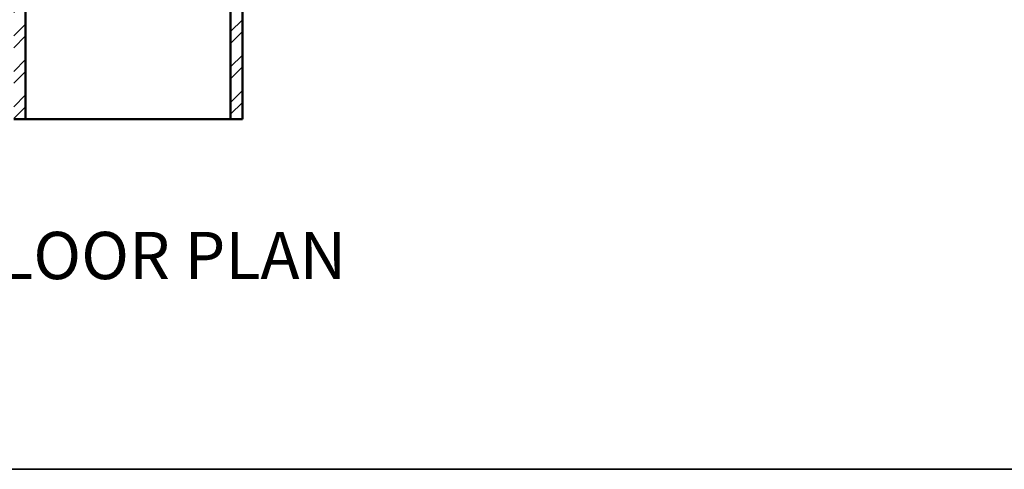
# Model space of a CAD drawing. Units: inches. Extents: x 963 to 2075, y 289 to 2657.
# Tile 30 of 98: x 1511 to 1885, y 1303 to 1474. Entities that reach past the tile are written whole.
import ezdxf

# ---------------------------------------------------------------- set-up
doc = ezdxf.new("R2010")
doc.units = ezdxf.units.IN
for name, color, linetype, lineweight in [('A-ANNO-TEXT', 7, 'Continuous', 25), ('A-ANNO-TTLB', 7, 'Continuous', 35), ('A-WALL', 7, 'Continuous', 50), ('A-WALL-PATT', 8, 'Continuous', 13)]:
    doc.layers.add(name, color=color, linetype=linetype, lineweight=lineweight)
doc.styles.get("Standard").update_dxf_attribs({"font": 'arial.ttf'})

msp = doc.modelspace()

# ---------------------------------------------------------------- hatches: boundary and pattern name
at = {"layer": 'A-WALL-PATT'}
h = msp.add_hatch(dxfattribs=at)
h.set_pattern_fill('ANSI32', color=256)
h.paths.add_polyline_path([(1296.92, 2558.32), (1203.92, 2558.32), (1203.92, 2493.82), (1191.53, 2493.82), (1191.53, 2489.32), (1211.06, 2489.32), (1211.06, 2492.02), (1211.06, 2493.82), (1208.42, 2493.82), (1208.42, 2553.82), (1292.42, 2553.82), (1292.42, 2538.86), (1296.92, 2538.86)])
h.paths.add_polyline_path([(1442.42, 2558.32), (1349.42, 2558.32), (1349.42, 2538.94), (1353.92, 2538.94), (1353.92, 2553.82), (1437.92, 2553.82), (1437.92, 2493.82), (1434.54, 2493.82), (1434.54, 2489.32), (1448.31, 2489.32), (1448.31, 2491.57), (1448.31, 2493.82), (1442.42, 2493.82)])
h.paths.add_polyline_path([(1415.55, 2491.57), (1415.55, 2493.82), (1340.94, 2493.82), (1340.94, 2489.32), (1371.92, 2489.32), (1371.92, 2378.32), (1367.6, 2378.32), (1367.6, 2373.82), (1371.92, 2373.82), (1371.92, 2355.19), (1376.42, 2355.19), (1376.42, 2489.32), (1415.55, 2489.32)])
h.paths.add_polyline_path([(1304.94, 2491.57), (1304.94, 2493.82), (1296.92, 2493.82), (1296.92, 2514.86), (1292.42, 2514.86), (1292.42, 2493.82), (1232.81, 2493.82), (1232.81, 2489.32), (1256.42, 2489.32), (1256.42, 2327.32), (1253.71, 2327.32), (1253.71, 2322.82), (1328.42, 2322.82), (1328.42, 2331.15), (1323.92, 2331.15), (1323.92, 2327.32), (1260.92, 2327.32), (1260.92, 2373.82), (1323.92, 2373.82), (1323.92, 2357.81), (1328.42, 2357.81), (1328.42, 2373.82), (1346.01, 2373.82), (1346.01, 2376.07), (1346.01, 2378.32), (1260.92, 2378.32), (1260.92, 2489.32), (1304.94, 2489.32)])
h.paths.add_polyline_path([(1226.65, 2327.32), (1124.42, 2327.32), (1124.42, 2347.45), (1119.92, 2347.45), (1119.92, 2322.82), (1163.42, 2322.82), (1163.42, 2305.43), (1165.67, 2305.43), (1167.92, 2305.43), (1167.92, 2322.82), (1226.65, 2322.82), (1226.65, 2325.07)])
h.paths.add_polyline_path([(1095.92, 2489.32), (1124.42, 2489.32), (1131.53, 2489.32), (1131.53, 2491.57), (1131.53, 2493.82), (1119.92, 2493.82), (1091.42, 2493.82), (1091.42, 2417.32), (1095.92, 2417.32), (1119.92, 2417.32), (1119.92, 2407.45), (1124.42, 2407.45), (1124.42, 2421.82), (1095.92, 2421.82)])
h.paths.add_polyline_path([(1512.92, 2558.32), (1508.42, 2558.32), (1508.42, 2493.82), (1503.4, 2493.82), (1503.4, 2489.32), (1508.42, 2489.32), (1508.42, 2327.32), (1376.42, 2327.32), (1376.42, 2330.27), (1371.92, 2330.27), (1371.92, 2298.74), (1376.42, 2298.74), (1376.42, 2322.82), (1508.42, 2322.82), (1508.42, 2165.32), (1504.26, 2165.32), (1504.26, 2160.82), (1508.42, 2160.82), (1508.42, 2108.32), (1512.92, 2108.32), (1512.92, 2160.82), (1516.18, 2160.82), (1516.18, 2163.07), (1516.18, 2165.32), (1512.92, 2165.32), (1512.92, 2322.82), (1644.92, 2322.82), (1644.92, 2298.74), (1649.42, 2298.74), (1649.42, 2322.82), (1649.42, 2330.94), (1647.17, 2330.94), (1644.92, 2330.94), (1644.92, 2327.32), (1512.92, 2327.32), (1512.92, 2489.32), (1516.76, 2489.32), (1516.76, 2491.57), (1516.76, 2493.82), (1512.92, 2493.82)])
h.paths.add_polyline_path([(1671.92, 2558.32), (1578.92, 2558.32), (1578.92, 2493.82), (1573.53, 2493.82), (1573.53, 2489.32), (1586.54, 2489.32), (1586.54, 2491.57), (1586.54, 2493.82), (1583.42, 2493.82), (1583.42, 2553.82), (1667.42, 2553.82), (1667.42, 2541.11), (1671.92, 2541.11)])
h.paths.add_polyline_path([(1681.26, 2493.82), (1671.92, 2493.82), (1671.92, 2517.11), (1667.42, 2517.11), (1667.42, 2493.82), (1610.22, 2493.82), (1610.22, 2489.32), (1644.92, 2489.32), (1644.92, 2357.87), (1649.42, 2357.87), (1649.42, 2373.82), (1652.2, 2373.82), (1652.2, 2375.83), (1652.2, 2378.32), (1649.42, 2378.32), (1649.42, 2489.32), (1681.26, 2489.32), (1681.26, 2491.57)])
h.paths.add_polyline_path([(1821.92, 2558.32), (1728.92, 2558.32), (1728.92, 2541), (1733.42, 2541), (1733.42, 2553.82), (1817.42, 2553.82), (1817.42, 2493.82), (1813.51, 2493.82), (1813.51, 2489.32), (1830.08, 2489.32), (1830.08, 2491.57), (1830.08, 2493.82), (1821.92, 2493.82)])
h.paths.add_polyline_path([(1794.24, 2493.82), (1717.26, 2493.82), (1717.26, 2489.32), (1760.42, 2489.32), (1760.42, 2378.32), (1674.4, 2378.32), (1674.4, 2373.82), (1692.92, 2373.82), (1692.92, 2356.95), (1697.42, 2356.95), (1697.42, 2373.82), (1760.42, 2373.82), (1760.42, 2327.32), (1697.42, 2327.32), (1697.42, 2333.34), (1692.92, 2333.34), (1692.92, 2322.82), (1768.04, 2322.82), (1768.04, 2325.07), (1768.04, 2327.32), (1764.92, 2327.32), (1764.92, 2489.32), (1794.24, 2489.32)])
h.paths.add_polyline_path([(1733.42, 2517), (1728.92, 2517), (1728.92, 2493.82), (1733.42, 2493.82)], flags=17)
h.paths.add_polyline_path([(1929.92, 2493.82), (1890.08, 2493.82), (1890.08, 2489.32), (1896.92, 2489.32), (1925.42, 2489.32), (1925.42, 2421.82), (1896.92, 2421.82), (1896.92, 2408.32), (1901.42, 2408.32), (1901.42, 2417.32), (1925.42, 2417.32), (1929.92, 2417.32)])
h.paths.add_polyline_path([(1901.42, 2348.32), (1896.92, 2348.32), (1896.92, 2327.32), (1800.42, 2327.32), (1800.42, 2322.82), (1853.42, 2322.82), (1853.42, 2309.45), (1857.92, 2309.45), (1857.92, 2322.82), (1901.42, 2322.82)])
h.paths.add_polyline_path([(1857.92, 2249.45), (1853.42, 2249.45), (1853.42, 2214.82), (1686.31, 2214.82), (1686.31, 2210.32), (1853.42, 2210.32), (1853.42, 2202.13), (1857.92, 2202.13), (1857.92, 2210.32)])
h.paths.add_polyline_path([(1857.92, 2142.13), (1853.42, 2142.13), (1853.42, 2115.42), (1841.42, 2115.42), (1841.42, 2088.53), (1841.42, 2046.95), (1845.92, 2046.95), (1845.92, 2110.92), (1905.92, 2110.92), (1905.92, 2092.52), (1910.42, 2092.52), (1910.42, 2115.42), (1857.92, 2115.42)])
h.paths.add_polyline_path([(1532.44, 1482.34), (1573.46, 1482.34), (1573.46, 1501), (1532.44, 1501)], flags=9)
h.paths.add_polyline_path([(1438.66, 1486.3), (1479.68, 1486.3), (1479.68, 1504.96), (1438.66, 1504.96)], flags=9)
h.paths.add_polyline_path([(1411.22, 1365.31), (1659.14, 1365.31), (1659.14, 1402.4), (1411.22, 1402.4)], flags=9)
h.paths.add_polyline_path([(1185.67, 2296.3), (1248.16, 2296.3), (1248.16, 2314.95), (1185.67, 2314.95)], flags=9)
h.paths.add_polyline_path([(1177.31, 2187.35), (1216.15, 2187.35), (1216.15, 2206.01), (1177.31, 2206.01)], flags=9)
h.paths.add_polyline_path([(1295.1, 1602.08), (1328.26, 1602.08), (1328.26, 1620.74), (1295.1, 1620.74)], flags=9)
h.paths.add_polyline_path([(1525.13, 2005.99), (1558.39, 2005.99), (1558.39, 2024.65), (1525.13, 2024.65)], flags=9)
h.paths.add_polyline_path([(1459.61, 1977.13), (1472.19, 1977.13), (1472.19, 1987.43), (1459.61, 1987.43)], flags=9)
h.paths.add_polyline_path([(1467.81, 2053.68), (1480.02, 2053.68), (1480.02, 2063.98), (1467.81, 2063.98)], flags=9)
h.paths.add_polyline_path([(1555.18, 2119.02), (1584.56, 2119.02), (1584.56, 2137.68), (1555.18, 2137.68)], flags=25)
h.paths.add_polyline_path([(1405.39, 2115.29), (1444.48, 2115.29), (1444.48, 2133.95), (1405.39, 2133.95)], flags=25)
h.paths.add_polyline_path([(1698.48, 2004.26), (1727.69, 2004.26), (1727.69, 2022.92), (1698.48, 2022.92)], flags=9)
h.paths.add_polyline_path([(1612.16, 1972.86), (1629.02, 1972.86), (1629.02, 1983.16), (1612.16, 1983.16)], flags=9)
h.paths.add_polyline_path([(1608.29, 2060.04), (1625.15, 2060.04), (1625.15, 2070.34), (1608.29, 2070.34)], flags=9)
h.paths.add_polyline_path([(1527.95, 1684.4), (1566.79, 1684.4), (1566.79, 1703.06), (1527.95, 1703.06)], flags=9)
h.paths.add_polyline_path([(1422.79, 1683.59), (1461.63, 1683.59), (1461.63, 1702.25), (1422.79, 1702.25)], flags=9)
h.paths.add_polyline_path([(1531.26, 1732.46), (1574.01, 1732.46), (1574.01, 1751.12), (1531.26, 1751.12)], flags=9)
h.paths.add_polyline_path([(1402.87, 1732.85), (1439.8, 1732.85), (1439.8, 1751.5), (1402.87, 1751.5)], flags=9)
h.paths.add_polyline_path([(1243.12, 1923.13), (1281.96, 1923.13), (1281.96, 1941.79), (1243.12, 1941.79)], flags=9)
h.paths.add_polyline_path([(1181.75, 1792.27), (1244.24, 1792.27), (1244.24, 1810.93), (1181.75, 1810.93)], flags=9)
h.paths.add_polyline_path([(1265.82, 1670.3), (1316.07, 1670.3), (1316.07, 1688.96), (1265.82, 1688.96)], flags=9)
h.paths.add_polyline_path([(1140.26, 1676.05), (1179.1, 1676.05), (1179.1, 1694.71), (1140.26, 1694.71)], flags=9)
h.paths.add_polyline_path([(1107.49, 1490.89), (1143.37, 1490.89), (1143.37, 1509.55), (1107.49, 1509.55)], flags=9)
h.paths.add_polyline_path([(1217.58, 1483.9), (1246.74, 1483.9), (1246.74, 1502.56), (1217.58, 1502.56)], flags=9)
h.paths.add_polyline_path([(1389.21, 1486.92), (1418.37, 1486.92), (1418.37, 1505.58), (1389.21, 1505.58)], flags=9)
h.paths.add_polyline_path([(1672.21, 1602.08), (1705.37, 1602.08), (1705.37, 1620.74), (1672.21, 1620.74)], flags=9)
h.paths.add_polyline_path([(1752.08, 1522.64), (1781.24, 1522.64), (1781.24, 1541.3), (1752.08, 1541.3)], flags=9)
h.paths.add_polyline_path([(1848.27, 1491.26), (1884.16, 1491.26), (1884.16, 1509.92), (1848.27, 1509.92)], flags=9)
h.paths.add_polyline_path([(1822.47, 1685.62), (1861.31, 1685.62), (1861.31, 1704.28), (1822.47, 1704.28)], flags=9)
h.paths.add_polyline_path([(1713.19, 1672.23), (1763.44, 1672.23), (1763.44, 1690.89), (1713.19, 1690.89)], flags=9)
h.paths.add_polyline_path([(1736.62, 1790.58), (1799.11, 1790.58), (1799.11, 1809.24), (1736.62, 1809.24)], flags=9)
h.paths.add_polyline_path([(1691.49, 1916.36), (1730.33, 1916.36), (1730.33, 1935.01), (1691.49, 1935.01)], flags=9)
h.paths.add_polyline_path([(1764.87, 1973.92), (1794.31, 1973.92), (1794.31, 1992.58), (1764.87, 1992.58)], flags=9)
h.paths.add_polyline_path([(1767.85, 2034.02), (1797.29, 2034.02), (1797.29, 2052.67), (1767.85, 2052.67)], flags=9)
h.paths.add_polyline_path([(1851.59, 2060.33), (1880.75, 2060.33), (1880.75, 2078.99), (1851.59, 2078.99)], flags=25)
h.paths.add_polyline_path([(1688.49, 2086.87), (1727.33, 2086.87), (1727.33, 2105.53), (1688.49, 2105.53)], flags=9)
h.paths.add_polyline_path([(1537.74, 2293.58), (1580.49, 2293.58), (1580.49, 2312.24), (1537.74, 2312.24)], flags=25)
h.paths.add_polyline_path([(1425.59, 2296.11), (1468.34, 2296.11), (1468.34, 2314.77), (1425.59, 2314.77)], flags=25)
h.paths.add_polyline_path([(1278.52, 2004.18), (1307.72, 2004.18), (1307.72, 2022.84), (1278.52, 2022.84)], flags=9)
h.paths.add_polyline_path([(1193.28, 1973.63), (1222.72, 1973.63), (1222.72, 1992.29), (1193.28, 1992.29)], flags=9)
h.paths.add_polyline_path([(1192.41, 2040.58), (1221.84, 2040.58), (1221.84, 2059.23), (1192.41, 2059.23)], flags=9)
h.paths.add_polyline_path([(1130.6, 1951.39), (1159.76, 1951.39), (1159.76, 1970.05), (1130.6, 1970.05)], flags=9)
h.paths.add_polyline_path([(1132.83, 2052.49), (1161.98, 2052.49), (1161.98, 2071.15), (1132.83, 2071.15)], flags=9)
h.paths.add_polyline_path([(1265.13, 2334.62), (1315.38, 2334.62), (1315.38, 2353.28), (1265.13, 2353.28)], flags=25)
h.paths.add_polyline_path([(1136.74, 2330.79), (1175.58, 2330.79), (1175.58, 2349.44), (1136.74, 2349.44)], flags=9)
h.paths.add_polyline_path([(1287.42, 2417.2), (1320.58, 2417.2), (1320.58, 2435.86), (1287.42, 2435.86)], flags=25)
h.paths.add_polyline_path([(1430.99, 2329.16), (1469.83, 2329.16), (1469.83, 2347.82), (1430.99, 2347.82)], flags=25)
h.paths.add_polyline_path([(1525.42, 2329.21), (1564.26, 2329.21), (1564.26, 2347.87), (1525.42, 2347.87)], flags=25)
h.paths.add_polyline_path([(1684.52, 2382.8), (1717.68, 2382.8), (1717.68, 2401.46), (1684.52, 2401.46)], flags=25)
h.paths.add_polyline_path([(1704.81, 2340.29), (1755.05, 2340.29), (1755.05, 2358.95), (1704.81, 2358.95)], flags=25)
h.paths.add_polyline_path([(1694.11, 2287.76), (1756.6, 2287.76), (1756.6, 2306.41), (1694.11, 2306.41)], flags=9)
h.paths.add_polyline_path([(1815.78, 2329.86), (1854.62, 2329.86), (1854.62, 2348.52), (1815.78, 2348.52)], flags=9)
h.paths.add_polyline_path([(1842.87, 2514.26), (1878.76, 2514.26), (1878.76, 2532.91), (1842.87, 2532.91)], flags=9)
h.paths.add_polyline_path([(1769.51, 2531.45), (1798.67, 2531.45), (1798.67, 2550.1), (1769.51, 2550.1)], flags=25)
h.paths.add_polyline_path([(1594.77, 2518.47), (1623.93, 2518.47), (1623.93, 2537.13), (1594.77, 2537.13)], flags=25)
h.paths.add_polyline_path([(1520.72, 2516.18), (1556.61, 2516.18), (1556.61, 2534.84), (1520.72, 2534.84)], flags=25)
h.paths.add_polyline_path([(1464.46, 2516.69), (1500.34, 2516.69), (1500.34, 2535.35), (1464.46, 2535.35)], flags=25)
h.paths.add_polyline_path([(1365.7, 2528.97), (1394.85, 2528.97), (1394.85, 2547.63), (1365.7, 2547.63)], flags=25)
h.paths.add_polyline_path([(1222.84, 2516.23), (1252, 2516.23), (1252, 2534.89), (1222.84, 2534.89)], flags=25)
h.paths.add_polyline_path([(1104.55, 2509.6), (1140.43, 2509.6), (1140.43, 2528.26), (1104.55, 2528.26)], flags=9)
h = msp.add_hatch(dxfattribs=at)
h.set_pattern_fill('ANSI32', color=256)
h.paths.add_polyline_path([(1335.97, 2212.57), (1335.97, 2214.82), (1167.92, 2214.82), (1167.92, 2245.43), (1163.42, 2245.43), (1163.42, 2210.32), (1163.42, 2194.81), (1167.92, 2194.81), (1167.92, 2210.32), (1335.97, 2210.32)])
h.paths.add_polyline_path([(1532.44, 1482.34), (1573.46, 1482.34), (1573.46, 1501), (1532.44, 1501)], flags=9)
h.paths.add_polyline_path([(1438.66, 1486.3), (1479.68, 1486.3), (1479.68, 1504.96), (1438.66, 1504.96)], flags=9)
h.paths.add_polyline_path([(1411.22, 1365.31), (1659.14, 1365.31), (1659.14, 1402.4), (1411.22, 1402.4)], flags=9)
h.paths.add_polyline_path([(1185.67, 2296.3), (1248.16, 2296.3), (1248.16, 2314.95), (1185.67, 2314.95)], flags=9)
h.paths.add_polyline_path([(1177.31, 2187.35), (1216.15, 2187.35), (1216.15, 2206.01), (1177.31, 2206.01)], flags=9)
h.paths.add_polyline_path([(1295.1, 1602.08), (1328.26, 1602.08), (1328.26, 1620.74), (1295.1, 1620.74)], flags=9)
h.paths.add_polyline_path([(1525.13, 2005.99), (1558.39, 2005.99), (1558.39, 2024.65), (1525.13, 2024.65)], flags=9)
h.paths.add_polyline_path([(1459.61, 1977.13), (1472.19, 1977.13), (1472.19, 1987.43), (1459.61, 1987.43)], flags=9)
h.paths.add_polyline_path([(1467.81, 2053.68), (1480.02, 2053.68), (1480.02, 2063.98), (1467.81, 2063.98)], flags=9)
h.paths.add_polyline_path([(1555.18, 2119.02), (1584.56, 2119.02), (1584.56, 2137.68), (1555.18, 2137.68)], flags=9)
h.paths.add_polyline_path([(1405.39, 2115.29), (1444.48, 2115.29), (1444.48, 2133.95), (1405.39, 2133.95)], flags=9)
h.paths.add_polyline_path([(1698.48, 2004.26), (1727.69, 2004.26), (1727.69, 2022.92), (1698.48, 2022.92)], flags=9)
h.paths.add_polyline_path([(1612.16, 1972.86), (1629.02, 1972.86), (1629.02, 1983.16), (1612.16, 1983.16)], flags=9)
h.paths.add_polyline_path([(1608.29, 2060.04), (1625.15, 2060.04), (1625.15, 2070.34), (1608.29, 2070.34)], flags=9)
h.paths.add_polyline_path([(1527.95, 1684.4), (1566.79, 1684.4), (1566.79, 1703.06), (1527.95, 1703.06)], flags=9)
h.paths.add_polyline_path([(1422.79, 1683.59), (1461.63, 1683.59), (1461.63, 1702.25), (1422.79, 1702.25)], flags=9)
h.paths.add_polyline_path([(1531.26, 1732.46), (1574.01, 1732.46), (1574.01, 1751.12), (1531.26, 1751.12)], flags=9)
h.paths.add_polyline_path([(1402.87, 1732.85), (1439.8, 1732.85), (1439.8, 1751.5), (1402.87, 1751.5)], flags=9)
h.paths.add_polyline_path([(1243.12, 1923.13), (1281.96, 1923.13), (1281.96, 1941.79), (1243.12, 1941.79)], flags=9)
h.paths.add_polyline_path([(1181.75, 1792.27), (1244.24, 1792.27), (1244.24, 1810.93), (1181.75, 1810.93)], flags=9)
h.paths.add_polyline_path([(1265.82, 1670.3), (1316.07, 1670.3), (1316.07, 1688.96), (1265.82, 1688.96)], flags=9)
h.paths.add_polyline_path([(1140.26, 1676.05), (1179.1, 1676.05), (1179.1, 1694.71), (1140.26, 1694.71)], flags=9)
h.paths.add_polyline_path([(1107.49, 1490.89), (1143.37, 1490.89), (1143.37, 1509.55), (1107.49, 1509.55)], flags=9)
h.paths.add_polyline_path([(1217.58, 1483.9), (1246.74, 1483.9), (1246.74, 1502.56), (1217.58, 1502.56)], flags=9)
h.paths.add_polyline_path([(1389.21, 1486.92), (1418.37, 1486.92), (1418.37, 1505.58), (1389.21, 1505.58)], flags=9)
h.paths.add_polyline_path([(1672.21, 1602.08), (1705.37, 1602.08), (1705.37, 1620.74), (1672.21, 1620.74)], flags=9)
h.paths.add_polyline_path([(1752.08, 1522.64), (1781.24, 1522.64), (1781.24, 1541.3), (1752.08, 1541.3)], flags=9)
h.paths.add_polyline_path([(1848.27, 1491.26), (1884.16, 1491.26), (1884.16, 1509.92), (1848.27, 1509.92)], flags=9)
h.paths.add_polyline_path([(1822.47, 1685.62), (1861.31, 1685.62), (1861.31, 1704.28), (1822.47, 1704.28)], flags=9)
h.paths.add_polyline_path([(1713.19, 1672.23), (1763.44, 1672.23), (1763.44, 1690.89), (1713.19, 1690.89)], flags=9)
h.paths.add_polyline_path([(1736.62, 1790.58), (1799.11, 1790.58), (1799.11, 1809.24), (1736.62, 1809.24)], flags=9)
h.paths.add_polyline_path([(1691.49, 1916.36), (1730.33, 1916.36), (1730.33, 1935.01), (1691.49, 1935.01)], flags=9)
h.paths.add_polyline_path([(1764.87, 1973.92), (1794.31, 1973.92), (1794.31, 1992.58), (1764.87, 1992.58)], flags=9)
h.paths.add_polyline_path([(1767.85, 2034.02), (1797.29, 2034.02), (1797.29, 2052.67), (1767.85, 2052.67)], flags=9)
h.paths.add_polyline_path([(1851.59, 2060.33), (1880.75, 2060.33), (1880.75, 2078.99), (1851.59, 2078.99)], flags=9)
h.paths.add_polyline_path([(1688.49, 2086.87), (1727.33, 2086.87), (1727.33, 2105.53), (1688.49, 2105.53)], flags=9)
h.paths.add_polyline_path([(1537.74, 2293.58), (1580.49, 2293.58), (1580.49, 2312.24), (1537.74, 2312.24)], flags=9)
h.paths.add_polyline_path([(1425.59, 2296.11), (1468.34, 2296.11), (1468.34, 2314.77), (1425.59, 2314.77)], flags=9)
h.paths.add_polyline_path([(1278.52, 2004.18), (1307.72, 2004.18), (1307.72, 2022.84), (1278.52, 2022.84)], flags=9)
h.paths.add_polyline_path([(1193.28, 1973.63), (1222.72, 1973.63), (1222.72, 1992.29), (1193.28, 1992.29)], flags=9)
h.paths.add_polyline_path([(1192.41, 2040.58), (1221.84, 2040.58), (1221.84, 2059.23), (1192.41, 2059.23)], flags=9)
h.paths.add_polyline_path([(1130.6, 1951.39), (1159.76, 1951.39), (1159.76, 1970.05), (1130.6, 1970.05)], flags=9)
h.paths.add_polyline_path([(1132.83, 2052.49), (1161.98, 2052.49), (1161.98, 2071.15), (1132.83, 2071.15)], flags=9)
h.paths.add_polyline_path([(1265.13, 2334.62), (1315.38, 2334.62), (1315.38, 2353.28), (1265.13, 2353.28)], flags=9)
h.paths.add_polyline_path([(1136.74, 2330.79), (1175.58, 2330.79), (1175.58, 2349.44), (1136.74, 2349.44)], flags=9)
h.paths.add_polyline_path([(1287.42, 2417.2), (1320.58, 2417.2), (1320.58, 2435.86), (1287.42, 2435.86)], flags=9)
h.paths.add_polyline_path([(1430.99, 2329.16), (1469.83, 2329.16), (1469.83, 2347.82), (1430.99, 2347.82)], flags=9)
h.paths.add_polyline_path([(1525.42, 2329.21), (1564.26, 2329.21), (1564.26, 2347.87), (1525.42, 2347.87)], flags=9)
h.paths.add_polyline_path([(1684.52, 2382.8), (1717.68, 2382.8), (1717.68, 2401.46), (1684.52, 2401.46)], flags=9)
h.paths.add_polyline_path([(1704.81, 2340.29), (1755.05, 2340.29), (1755.05, 2358.95), (1704.81, 2358.95)], flags=9)
h.paths.add_polyline_path([(1694.11, 2287.76), (1756.6, 2287.76), (1756.6, 2306.41), (1694.11, 2306.41)], flags=9)
h.paths.add_polyline_path([(1815.78, 2329.86), (1854.62, 2329.86), (1854.62, 2348.52), (1815.78, 2348.52)], flags=9)
h.paths.add_polyline_path([(1842.87, 2514.26), (1878.76, 2514.26), (1878.76, 2532.91), (1842.87, 2532.91)], flags=9)
h.paths.add_polyline_path([(1769.51, 2531.45), (1798.67, 2531.45), (1798.67, 2550.1), (1769.51, 2550.1)], flags=9)
h.paths.add_polyline_path([(1594.77, 2518.47), (1623.93, 2518.47), (1623.93, 2537.13), (1594.77, 2537.13)], flags=9)
h.paths.add_polyline_path([(1520.72, 2516.18), (1556.61, 2516.18), (1556.61, 2534.84), (1520.72, 2534.84)], flags=9)
h.paths.add_polyline_path([(1464.46, 2516.69), (1500.34, 2516.69), (1500.34, 2535.35), (1464.46, 2535.35)], flags=9)
h.paths.add_polyline_path([(1365.7, 2528.97), (1394.85, 2528.97), (1394.85, 2547.63), (1365.7, 2547.63)], flags=9)
h.paths.add_polyline_path([(1222.84, 2516.23), (1252, 2516.23), (1252, 2534.89), (1222.84, 2534.89)], flags=9)
h.paths.add_polyline_path([(1104.55, 2509.6), (1140.43, 2509.6), (1140.43, 2528.26), (1104.55, 2528.26)], flags=9)
h = msp.add_hatch(dxfattribs=at)
h.set_pattern_fill('ANSI32', color=256)
h.paths.add_polyline_path([(1473.61, 2163.07), (1473.61, 2165.32), (1376.42, 2165.32), (1376.42, 2227.98), (1371.92, 2227.98), (1371.92, 2214.82), (1368.41, 2214.82), (1368.41, 2210.32), (1371.92, 2210.32), (1371.92, 2160.82), (1395.92, 2160.82), (1395.92, 2090.32), (1217.34, 2090.32), (1217.34, 2085.82), (1395.92, 2085.82), (1458.92, 2085.82), (1458.92, 2108.32), (1454.42, 2108.32), (1454.42, 2090.32), (1400.42, 2090.32), (1400.42, 2160.82), (1473.61, 2160.82)])
h.paths.add_polyline_path([(1649.42, 2210.32), (1653.23, 2210.32), (1653.23, 2214.82), (1649.42, 2214.82), (1649.42, 2227.98), (1644.92, 2227.98), (1644.92, 2165.32), (1550.1, 2165.32), (1550.1, 2160.82), (1620.92, 2160.82), (1620.92, 2112.82), (1555.45, 2112.82), (1555.45, 2108.32), (1584.33, 2108.32), (1584.33, 2084.92), (1588.83, 2084.92), (1588.83, 2108.32), (1625.42, 2108.32), (1667.95, 2108.32), (1667.95, 2022.67), (1588.83, 2022.67), (1588.83, 2047.41), (1584.33, 2047.41), (1584.33, 1996), (1588.83, 1996), (1588.83, 2018.32), (1667.95, 2018.17), (1667.95, 1928.32), (1625.42, 1928.32), (1625.42, 1923.82), (1672.45, 1923.82), (1672.45, 1928.32), (1672.45, 1946.66), (1785.45, 1946.66), (1785.45, 1951.16), (1743.03, 1951.16), (1743.03, 2017.92), (1841.42, 2017.92), (1841.42, 2014.77), (1845.92, 2014.77), (1845.92, 2017.92), (1905.92, 2017.92), (1905.92, 1987.51), (1910.42, 1987.51), (1910.42, 2022.42), (1910.42, 2068.52), (1905.92, 2068.52), (1905.92, 2022.42), (1845.92, 2022.42), (1845.92, 2025.85), (1843.67, 2025.85), (1841.42, 2025.85), (1841.42, 2022.42), (1743.03, 2022.42), (1743.03, 2084.03), (1768.45, 2084.03), (1785.45, 2084.03), (1785.45, 2088.53), (1672.45, 2088.53), (1672.45, 2112.82), (1667.95, 2112.82), (1625.42, 2112.82), (1625.42, 2160.82), (1649.42, 2160.82)])
h.paths.add_polyline_path([(1672.45, 2084.03), (1738.53, 2084.03), (1738.53, 1951.16), (1672.45, 1951.16)], flags=16)
h.paths.add_polyline_path([(1672.45, 2084.03), (1738.53, 2084.03), (1705.49, 2017.6)], flags=0)
h.paths.add_polyline_path([(1262.77, 2085.82), (1258.27, 2085.82), (1258.27, 2023.28), (1184.42, 2023.28), (1184.42, 2018.78), (1258.27, 2018.78), (1258.27, 1950.82), (1262.77, 1950.82)])
h.paths.add_polyline_path([(1312.27, 2085.82), (1307.77, 2085.82), (1307.77, 1950.82), (1312.27, 1950.82)])
h.paths.add_polyline_path([(1458.92, 1950.82), (1395.92, 1950.82), (1216.57, 1950.82), (1216.57, 1946.32), (1346.42, 1946.32), (1395.92, 1946.32), (1395.92, 1875.82), (1371.92, 1875.82), (1371.92, 1826.32), (1368.93, 1826.32), (1368.93, 1821.82), (1371.92, 1821.82), (1371.92, 1813.62), (1376.42, 1813.62), (1376.42, 1871.32), (1474.5, 1871.32), (1474.5, 1873.57), (1474.5, 1875.82), (1400.42, 1875.82), (1400.42, 1946.32), (1454.42, 1946.32), (1454.42, 1928.32), (1458.92, 1928.32)])
h.paths.add_polyline_path([(1184.42, 2120.78), (1167.92, 2120.78), (1167.92, 2134.81), (1165.67, 2134.81), (1163.42, 2134.81), (1163.42, 2120.78), (1119.92, 2120.78), (1119.92, 2098.1), (1124.42, 2098.1), (1124.42, 2116.28), (1167.92, 2116.28), (1179.92, 2116.28), (1179.92, 2045.92), (1184.42, 2045.92), (1184.42, 2090.32), (1184.42, 2116.28)])
h.paths.add_polyline_path([(1124.42, 2018.78), (1179.92, 2018.78), (1179.92, 2016.29), (1184.42, 2016.29), (1184.42, 2023.28), (1184.42, 2026.59), (1182.17, 2026.59), (1179.92, 2026.59), (1179.92, 2023.28), (1124.42, 2023.28), (1124.42, 2074.1), (1119.92, 2074.1), (1119.92, 2018.78), (1119.92, 1979.63), (1124.42, 1979.63)])
h.paths.add_polyline_path([(1184.42, 1925.78), (1184.42, 1946.32), (1184.42, 1996.07), (1182.17, 1996.07), (1179.92, 1996.07), (1179.92, 1925.78), (1124.42, 1925.78), (1124.42, 1955.63), (1119.92, 1955.5), (1119.92, 1921.28), (1158.92, 1921.28), (1158.92, 1909.98), (1163.42, 1909.98), (1163.42, 1921.28), (1184.42, 1921.28)])
h.paths.add_polyline_path([(1341.45, 1826.32), (1163.42, 1826.32), (1163.42, 1849.98), (1158.92, 1849.98), (1158.92, 1821.82), (1158.92, 1804.03), (1163.42, 1804.03), (1163.42, 1821.82), (1341.45, 1821.82)])
h.paths.add_polyline_path([(1222.98, 1713.82), (1163.42, 1713.82), (1163.42, 1744.03), (1161.17, 1744.03), (1158.92, 1744.03), (1158.92, 1713.82), (1119.92, 1713.82), (1119.92, 1694.65), (1124.42, 1694.65), (1124.42, 1709.32), (1158.92, 1709.32), (1222.98, 1709.32)])
h.paths.add_polyline_path([(1328.42, 1713.82), (1252.04, 1713.82), (1252.04, 1711.57), (1252.04, 1709.32), (1256.42, 1709.32), (1256.42, 1547.32), (1232.94, 1547.32), (1232.94, 1545.07), (1232.94, 1542.82), (1292.42, 1542.82), (1292.42, 1527.63), (1296.92, 1527.63), (1296.92, 1542.82), (1299.46, 1542.82), (1299.46, 1547.32), (1260.92, 1547.32), (1260.92, 1658.32), (1343.66, 1658.32), (1343.66, 1660.57), (1343.66, 1662.82), (1328.42, 1662.82), (1328.42, 1676.59), (1327.4, 1676.59), (1323.92, 1676.59), (1323.92, 1662.82), (1260.92, 1662.82), (1260.92, 1709.32), (1323.92, 1709.32), (1323.92, 1699.85), (1328.42, 1699.85)])
h.paths.add_polyline_path([(1649.42, 1875.82), (1625.42, 1875.82), (1625.42, 1928.32), (1620.92, 1928.32), (1588.83, 1928.32), (1588.83, 1950.59), (1584.33, 1950.59), (1584.33, 1928.32), (1555.45, 1928.32), (1555.45, 1923.82), (1620.92, 1923.82), (1620.92, 1875.82), (1548.95, 1875.82), (1548.95, 1873.57), (1548.95, 1871.32), (1644.92, 1871.32), (1644.92, 1813.62), (1649.42, 1813.62), (1649.42, 1821.82), (1652.04, 1821.82), (1652.04, 1824.07), (1652.04, 1826.32), (1649.42, 1826.32)])
h.paths.add_polyline_path([(1512.92, 1871.32), (1516.48, 1871.32), (1516.48, 1875.82), (1512.92, 1875.82), (1512.92, 1923.82), (1512.92, 1928.32), (1512.92, 1930.83), (1508.42, 1930.83), (1508.42, 1875.82), (1504.41, 1875.82), (1504.41, 1871.32), (1508.42, 1871.32), (1508.42, 1713.82), (1376.42, 1713.82), (1376.42, 1743.32), (1371.92, 1743.32), (1371.92, 1709.32), (1371.92, 1706.01), (1376.42, 1706.01), (1376.42, 1709.32), (1508.42, 1709.32), (1508.42, 1547.32), (1501.87, 1547.32), (1501.87, 1542.82), (1508.42, 1542.82), (1508.42, 1482.82), (1508.42, 1436.32), (1512.92, 1436.32), (1512.92, 1542.82), (1519.32, 1542.82), (1519.32, 1545.07), (1519.32, 1547.32), (1512.92, 1547.32), (1512.92, 1709.32), (1644.92, 1709.32), (1644.92, 1707.55), (1649.42, 1707.55), (1649.42, 1709.32), (1649.42, 1743.32), (1644.92, 1743.32), (1644.92, 1713.82), (1512.92, 1713.82)])
h.paths.add_polyline_path([(1129.88, 1545.07), (1129.88, 1547.32), (1124.42, 1547.32), (1095.92, 1547.32), (1095.92, 1614.82), (1124.42, 1614.82), (1124.42, 1619.32), (1095.92, 1619.32), (1091.42, 1619.32), (1091.42, 1542.82), (1095.92, 1542.82), (1119.92, 1542.82), (1129.88, 1542.82)])
h.paths.add_polyline_path([(1208.42, 1542.82), (1211.74, 1542.82), (1211.74, 1547.32), (1198.85, 1547.32), (1198.85, 1542.82), (1203.92, 1542.82), (1203.92, 1478.32), (1208.42, 1478.32), (1296.92, 1478.32), (1296.92, 1503.63), (1292.42, 1503.63), (1292.42, 1482.82), (1208.42, 1482.82)])
h.paths.add_polyline_path([(1430.42, 1542.82), (1435.7, 1542.82), (1435.7, 1545.07), (1435.7, 1547.32), (1422.66, 1547.32), (1422.66, 1545.07), (1422.66, 1542.82), (1425.92, 1542.82), (1425.92, 1482.86), (1341.92, 1482.86), (1341.92, 1502.73), (1337.42, 1502.73), (1337.42, 1478.36), (1425.92, 1478.36), (1425.92, 1440.82), (1425.92, 1436.32), (1430.42, 1436.32)])
h.paths.add_polyline_path([(1698.48, 2004.26), (1727.69, 2004.26), (1727.69, 2022.92), (1698.48, 2022.92)], flags=8)
h = msp.add_hatch(dxfattribs=at)
h.set_pattern_fill('ANSI32', color=256)
h.paths.add_polyline_path([(1910.42, 1929.42), (1910.42, 1963.51), (1905.92, 1963.51), (1905.92, 1929.42), (1845.92, 1929.42), (1845.92, 1993.37), (1843.67, 1993.37), (1841.42, 1993.37), (1841.42, 1951.16), (1841.42, 1924.92), (1853.42, 1924.92), (1853.42, 1913.07), (1857.92, 1913.07), (1857.92, 1924.92), (1910.42, 1924.92)])
h.paths.add_polyline_path([(1857.92, 1853.07), (1853.42, 1853.07), (1853.42, 1826.32), (1841.42, 1826.32), (1674.48, 1826.32), (1674.48, 1821.82), (1853.42, 1821.82), (1857.92, 1821.82)])
h.paths.add_polyline_path([(1857.92, 1821.82), (1853.42, 1821.82), (1853.42, 1807.79), (1857.92, 1807.79)])
h.paths.add_polyline_path([(1857.92, 1747.79), (1853.42, 1747.79), (1853.42, 1713.82), (1809.34, 1713.82), (1809.34, 1709.32), (1905.92, 1709.32), (1905.92, 1688.32), (1910.42, 1688.32), (1910.42, 1713.82), (1857.92, 1713.82)])
h.paths.add_polyline_path([(1830.92, 1542.82), (1837.43, 1542.82), (1837.43, 1545.07), (1837.43, 1547.32), (1823.42, 1547.32), (1823.42, 1545.07), (1823.42, 1542.82), (1826.42, 1542.82), (1826.42, 1482.82), (1742.42, 1482.82), (1742.42, 1505.39), (1737.92, 1505.39), (1737.92, 1478.32), (1830.92, 1478.32)])
h.paths.add_polyline_path([(1938.92, 1619.32), (1934.42, 1619.32), (1910.42, 1619.32), (1910.42, 1628.32), (1908.17, 1628.32), (1905.92, 1628.32), (1905.92, 1614.82), (1934.42, 1614.82), (1934.42, 1547.32), (1905.92, 1547.32), (1899.59, 1547.32), (1899.59, 1542.82), (1910.42, 1542.82), (1938.92, 1542.82)])
h.paths.add_polyline_path([(1803.68, 1547.32), (1773.92, 1547.32), (1773.92, 1709.32), (1777.76, 1709.32), (1777.76, 1713.82), (1701.92, 1713.82), (1701.92, 1697.8), (1706.42, 1697.8), (1706.42, 1709.32), (1769.42, 1709.32), (1769.42, 1662.82), (1706.42, 1662.82), (1706.42, 1674.38), (1701.92, 1674.38), (1701.92, 1662.82), (1675.67, 1662.82), (1675.67, 1658.32), (1769.42, 1658.32), (1769.42, 1547.32), (1729.17, 1547.32), (1729.17, 1542.82), (1737.92, 1542.82), (1737.92, 1529.39), (1742.42, 1529.39), (1742.42, 1542.82), (1803.68, 1542.82)])
h.paths.add_polyline_path([(1595.42, 1542.82), (1599.24, 1542.82), (1599.24, 1547.32), (1584.36, 1547.32), (1584.36, 1542.82), (1590.92, 1542.82), (1590.92, 1436.32), (1595.42, 1436.32), (1595.42, 1440.82)])
h.paths.add_polyline_path([(1693.17, 1547.32), (1649.42, 1547.32), (1649.42, 1658.32), (1652.1, 1658.32), (1652.1, 1660.57), (1652.1, 1662.82), (1649.42, 1662.82), (1649.42, 1680.94), (1647.17, 1680.94), (1644.92, 1680.94), (1644.92, 1547.32), (1622.42, 1547.32), (1622.42, 1545.07), (1622.42, 1542.82), (1649.42, 1542.82), (1679.42, 1542.82), (1679.42, 1529.85), (1681.67, 1529.85), (1683.92, 1529.85), (1683.92, 1542.82), (1693.17, 1542.82), (1693.17, 1545.07)])
h.paths.add_polyline_path([(1683.92, 1505.85), (1679.42, 1505.85), (1679.42, 1483.8), (1595.42, 1483.8), (1595.42, 1479.3), (1683.92, 1479.3)])
h.paths.add_polyline_path([(1402.99, 1547.32), (1376.42, 1547.32), (1376.42, 1675.89), (1374.17, 1675.89), (1371.92, 1675.89), (1371.92, 1662.82), (1368.88, 1662.82), (1368.88, 1658.32), (1371.92, 1658.32), (1371.92, 1547.32), (1335.46, 1547.32), (1335.46, 1542.82), (1337.42, 1542.82), (1337.42, 1526.73), (1341.92, 1526.73), (1341.92, 1542.82), (1371.92, 1542.82), (1402.99, 1542.82)])

# ---------------------------------------------------------------- linework, layer by layer
at = {"layer": 'A-ANNO-TTLB'}
msp.add_lwpolyline([(962.81, 2657.49), (2074.6, 2657.49), (2074.6, 1303.08), (962.81, 1303.08)], close=True, dxfattribs=at)
at = {"layer": 'A-WALL'}
for p, q in [((1512.92, 1542.82), (1512.92, 1436.32)), ((1590.92, 1436.32), (1590.92, 1542.82)), ((1595.42, 1542.82), (1595.42, 1440.82)), ((1595.42, 1440.82), (1595.42, 1436.32)), ((1512.92, 1436.32), (1508.42, 1436.32)), ((1595.42, 1436.32), (1512.92, 1436.32))]:
    msp.add_line(p, q, dxfattribs=at)

# ---------------------------------------------------------------- texts
at = {"layer": 'A-ANNO-TEXT', "insert": (1417.78, 1393.46), "char_height": 18, "attachment_point": 1}
msp.add_mtext_dynamic_manual_height_columns('FIRST FLOOR PLAN ', width=783.3157, gutter_width=12.5, heights=[0], dxfattribs=at)

doc.saveas('drawing.dxf')
